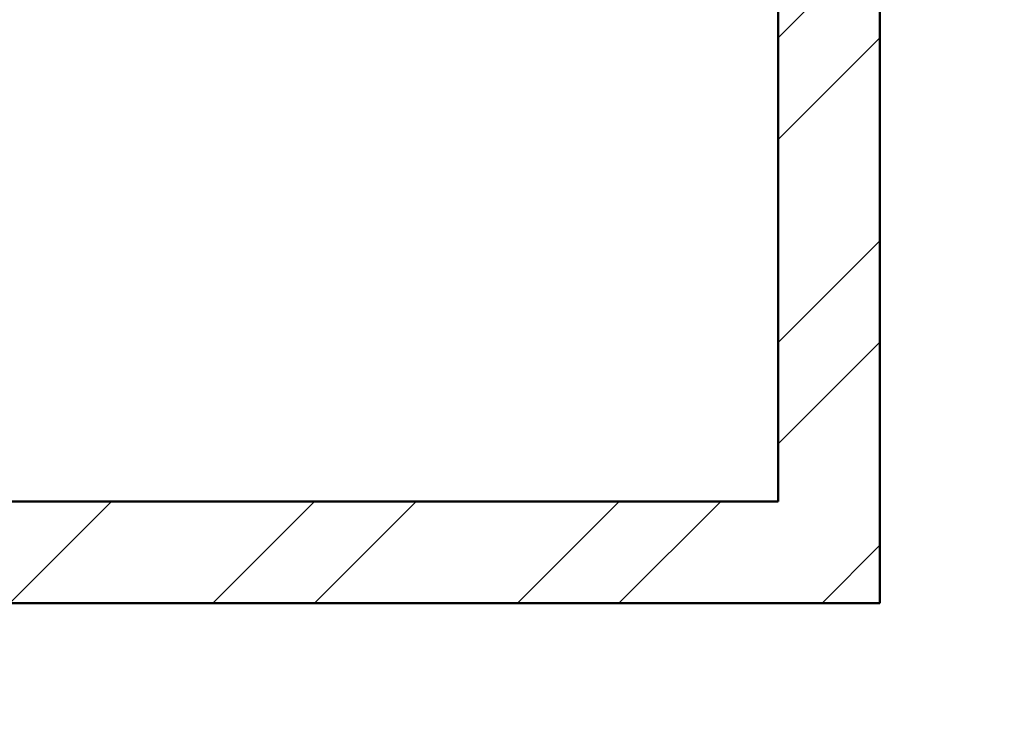
# Model space of a CAD drawing. Units: inches. Extents: x 963 to 2075, y 289 to 2657.
# Tile 33 of 98: x 1646 to 1689, y 1474 to 1505. Entities that reach past the tile are written whole.
import ezdxf

# ---------------------------------------------------------------- set-up
doc = ezdxf.new("R2010")
doc.units = ezdxf.units.IN
doc.layers.add('A-WALL', color=7, linetype='Continuous', lineweight=50)
doc.layers.add('A-WALL-PATT', color=8, linetype='Continuous', lineweight=13)

msp = doc.modelspace()

# ---------------------------------------------------------------- hatches: boundary and pattern name
at = {"layer": 'A-WALL-PATT'}
h = msp.add_hatch(dxfattribs=at)
h.set_pattern_fill('ANSI32', color=256)
h.paths.add_polyline_path([(1910.422, 1929.422), (1910.422, 1963.511), (1905.922, 1963.511), (1905.922, 1929.422), (1845.922, 1929.422), (1845.922, 1993.365), (1843.672, 1993.365), (1841.422, 1993.365), (1841.422, 1951.163), (1841.422, 1924.922), (1853.422, 1924.922), (1853.422, 1913.074), (1857.922, 1913.074), (1857.922, 1924.922), (1910.422, 1924.922)])
h.paths.add_polyline_path([(1857.922, 1853.074), (1853.422, 1853.074), (1853.422, 1826.318), (1841.422, 1826.318), (1674.482, 1826.318), (1674.482, 1821.818), (1853.422, 1821.818), (1857.922, 1821.818)])
h.paths.add_polyline_path([(1857.922, 1821.818), (1853.422, 1821.818), (1853.422, 1807.793), (1857.922, 1807.793)])
h.paths.add_polyline_path([(1857.922, 1747.793), (1853.422, 1747.793), (1853.422, 1713.818), (1809.343, 1713.818), (1809.343, 1709.318), (1905.922, 1709.318), (1905.922, 1688.318), (1910.422, 1688.318), (1910.422, 1713.818), (1857.922, 1713.818)])
h.paths.add_polyline_path([(1830.922, 1542.818), (1837.429, 1542.818), (1837.429, 1545.068), (1837.429, 1547.318), (1823.419, 1547.318), (1823.419, 1545.068), (1823.419, 1542.818), (1826.422, 1542.818), (1826.422, 1482.818), (1742.422, 1482.818), (1742.422, 1505.389), (1737.922, 1505.389), (1737.922, 1478.318), (1830.922, 1478.318)])
h.paths.add_polyline_path([(1938.922, 1619.318), (1934.422, 1619.318), (1910.422, 1619.318), (1910.422, 1628.318), (1908.172, 1628.318), (1905.922, 1628.318), (1905.922, 1614.818), (1934.422, 1614.818), (1934.422, 1547.318), (1905.922, 1547.318), (1899.589, 1547.318), (1899.589, 1542.818), (1910.422, 1542.818), (1938.922, 1542.818)])
h.paths.add_polyline_path([(1803.676, 1547.318), (1773.922, 1547.318), (1773.922, 1709.318), (1777.757, 1709.318), (1777.757, 1713.818), (1701.922, 1713.818), (1701.922, 1697.802), (1706.422, 1697.802), (1706.422, 1709.318), (1769.422, 1709.318), (1769.422, 1662.818), (1706.422, 1662.818), (1706.422, 1674.385), (1701.922, 1674.385), (1701.922, 1662.818), (1675.672, 1662.818), (1675.672, 1658.318), (1769.422, 1658.318), (1769.422, 1547.318), (1729.17, 1547.318), (1729.17, 1542.818), (1737.922, 1542.818), (1737.922, 1529.389), (1742.422, 1529.389), (1742.422, 1542.818), (1803.676, 1542.818)])
h.paths.add_polyline_path([(1595.422, 1542.818), (1599.245, 1542.818), (1599.245, 1547.318), (1584.36, 1547.318), (1584.36, 1542.818), (1590.922, 1542.818), (1590.922, 1436.318), (1595.422, 1436.318), (1595.422, 1440.818)])
h.paths.add_polyline_path([(1693.17, 1547.318), (1649.422, 1547.318), (1649.422, 1658.318), (1652.098, 1658.318), (1652.098, 1660.568), (1652.098, 1662.818), (1649.422, 1662.818), (1649.422, 1680.937), (1647.172, 1680.937), (1644.922, 1680.937), (1644.922, 1547.318), (1622.422, 1547.318), (1622.422, 1545.068), (1622.422, 1542.818), (1649.422, 1542.818), (1679.422, 1542.818), (1679.422, 1529.845), (1681.672, 1529.845), (1683.922, 1529.845), (1683.922, 1542.818), (1693.17, 1542.818), (1693.17, 1545.068)])
h.paths.add_polyline_path([(1683.922, 1505.845), (1679.422, 1505.845), (1679.422, 1483.805), (1595.422, 1483.805), (1595.422, 1479.305), (1683.922, 1479.305)])
h.paths.add_polyline_path([(1402.993, 1547.318), (1376.422, 1547.318), (1376.422, 1675.888), (1374.172, 1675.888), (1371.922, 1675.888), (1371.922, 1662.818), (1368.876, 1662.818), (1368.876, 1658.318), (1371.922, 1658.318), (1371.922, 1547.318), (1335.464, 1547.318), (1335.464, 1542.818), (1337.422, 1542.818), (1337.422, 1526.732), (1341.922, 1526.732), (1341.922, 1542.818), (1371.922, 1542.818), (1402.993, 1542.818)])

# ---------------------------------------------------------------- linework, layer by layer
at = {"layer": 'A-WALL'}
for p, q in [((1679.422, 1505.845), (1679.422, 1483.805)), ((1683.922, 1505.845), (1683.922, 1479.305)), ((1679.422, 1483.805), (1595.422, 1483.805)), ((1595.422, 1479.305), (1683.922, 1479.305))]:
    msp.add_line(p, q, dxfattribs=at)

doc.saveas('drawing.dxf')
